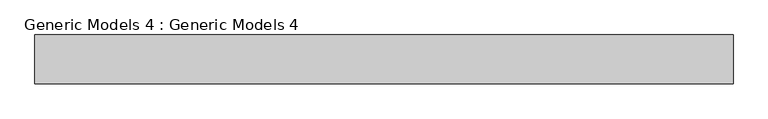
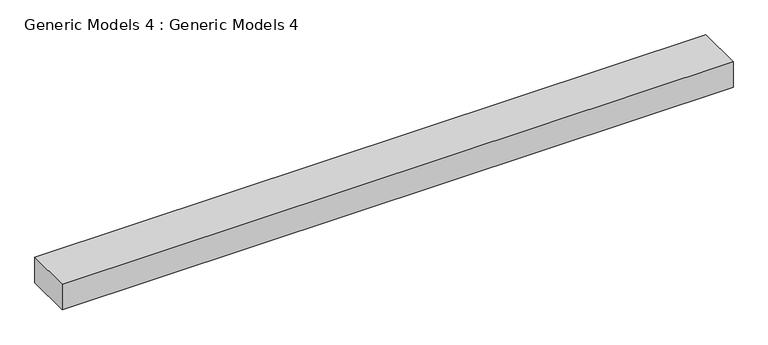
"""IFC4 building model written with IfcOpenShell, lengths in millimetres: proxy geometry, Generic Models 4 : Generic Models 4."""

from ifc_helpers import new_model, si_unit, frame, origin, place, context, project, spatial, polyline, outline, extrude, source, transform, mapped, element, save


def generic_models_4_generic_models_4_bf47a03a(model_context):
    return source(origin(), model_context, "Body", "SweptSolid", [
        extrude(outline(polyline([(-1332.7388314, 1851.619734), (-1332.7388314, 1235.5282073), (-10121.214981, 1235.5282073), (-10121.214981, 1851.619734), (-1332.7388314, 1851.619734)])), frame((0.0, 0.0, 6219.0690799), z_axis=(0.0, 0.0, 1.0), x_axis=(1.0, 0.0, 0.0)), (0.0, 0.0, 1.0), 354.3488304),
    ])


if __name__ == "__main__":
    model = new_model("IFC4")
    model_context = context("Model", 3, world=origin())
    ifc_project = project(units=[si_unit("LENGTHUNIT", "METRE", prefix="MILLI")], contexts=[model_context])
    site = spatial("IfcSite", under=ifc_project)
    building = spatial("IfcBuilding", under=site)
    placement = place(None, origin())
    generic_models_4_generic_models_4_shape = generic_models_4_generic_models_4_bf47a03a(model_context)
    element("IfcBuildingElementProxy", 1, Name="Generic Models 4 : Generic Models 4", ObjectType="Generic Models 4 : Generic Models 4", at=placement, inside=building, context=model_context, shape_type="MappedRepresentation", body=[
        mapped(generic_models_4_generic_models_4_shape, transform((0.0, 0.0, 0.0), x_axis=(1.0, 0.0, 0.0), y_axis=(0.0, 1.0, 0.0), z_axis=(0.0, 0.0, 1.0))),
    ])
    save(model, "model.ifc")
